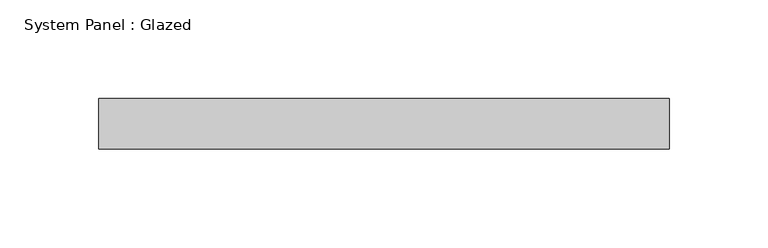
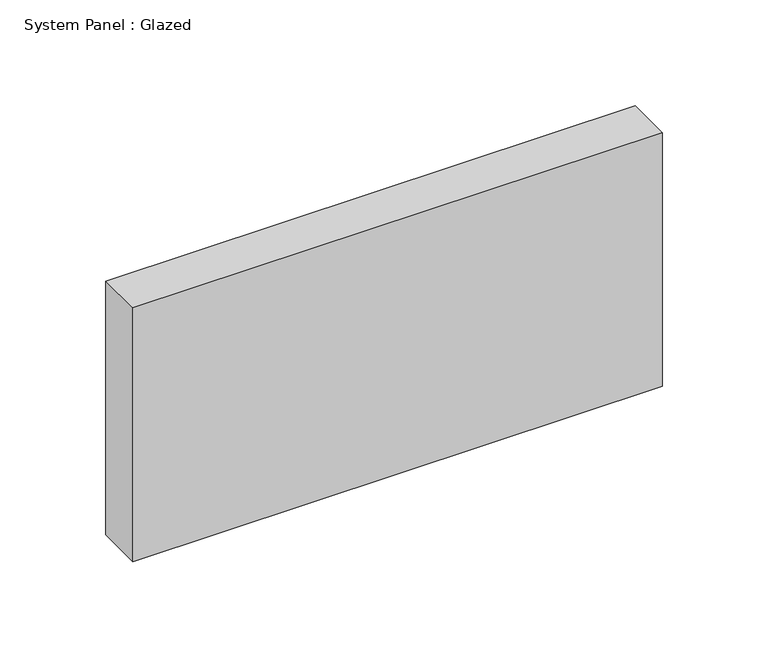
"""IFC4 building model written with IfcOpenShell, lengths in millimetres: plate geometry, System Panel : Glazed."""

from ifc_helpers import new_model, si_unit, origin, origin_with_axes, place, context, project, spatial, polyline, outline, extrude, source, transform, mapped, element, save


def system_panel_glazed_58d257f9(model_context):
    return source(origin(), model_context, "Body", "SweptSolid", [
        extrude(outline(polyline([(144.1160334, 19.05), (-144.1160334, 19.05), (-144.1160334, 44.45), (144.1160334, 44.45), (144.1160334, 19.05)])), origin_with_axes(), (0.0, 0.0, 1.0), 146.05),
    ])


if __name__ == "__main__":
    model = new_model("IFC4")
    model_context = context("Model", 3, world=origin())
    ifc_project = project(units=[si_unit("LENGTHUNIT", "METRE", prefix="MILLI")], contexts=[model_context])
    site = spatial("IfcSite", under=ifc_project)
    building = spatial("IfcBuilding", under=site)
    placement = place(None, origin())
    system_panel_glazed_shape = system_panel_glazed_58d257f9(model_context)
    element("IfcPlate", 1, ObjectType="System Panel : Glazed", at=placement, inside=building, context=model_context, shape_type="MappedRepresentation", body=[
        mapped(system_panel_glazed_shape, transform((0.0, 0.0, 0.0), x_axis=(1.0, 0.0, 0.0), y_axis=(0.0, 1.0, 0.0), z_axis=(0.0, 0.0, 1.0))),
    ])
    save(model, "model.ifc")

# Revit data of these elements
# Type "System Panel : Glazed"
#   Construction Type Id = "GSP4R"
#   Analytic Construction = "1/8 in Pilkington single glazing"
#   Visual Light Transmittance = 0.9
#   Solar Heat Gain Coefficient = 0.86
#   Heat Transfer Coefficient (U) = 1.18115 BTU/(h·ft²·°F)
#   Define Thermal Properties by = 1
# Element 1 (IfcPlate, "System Panel : Glazed")
#   Materials on its faces: "Glass"
# Materials
#   "Glass": class "Glass", colour RGB 0 128 192, transparency 0.75, Description = "Soda Lime Glass", Cost = 0
